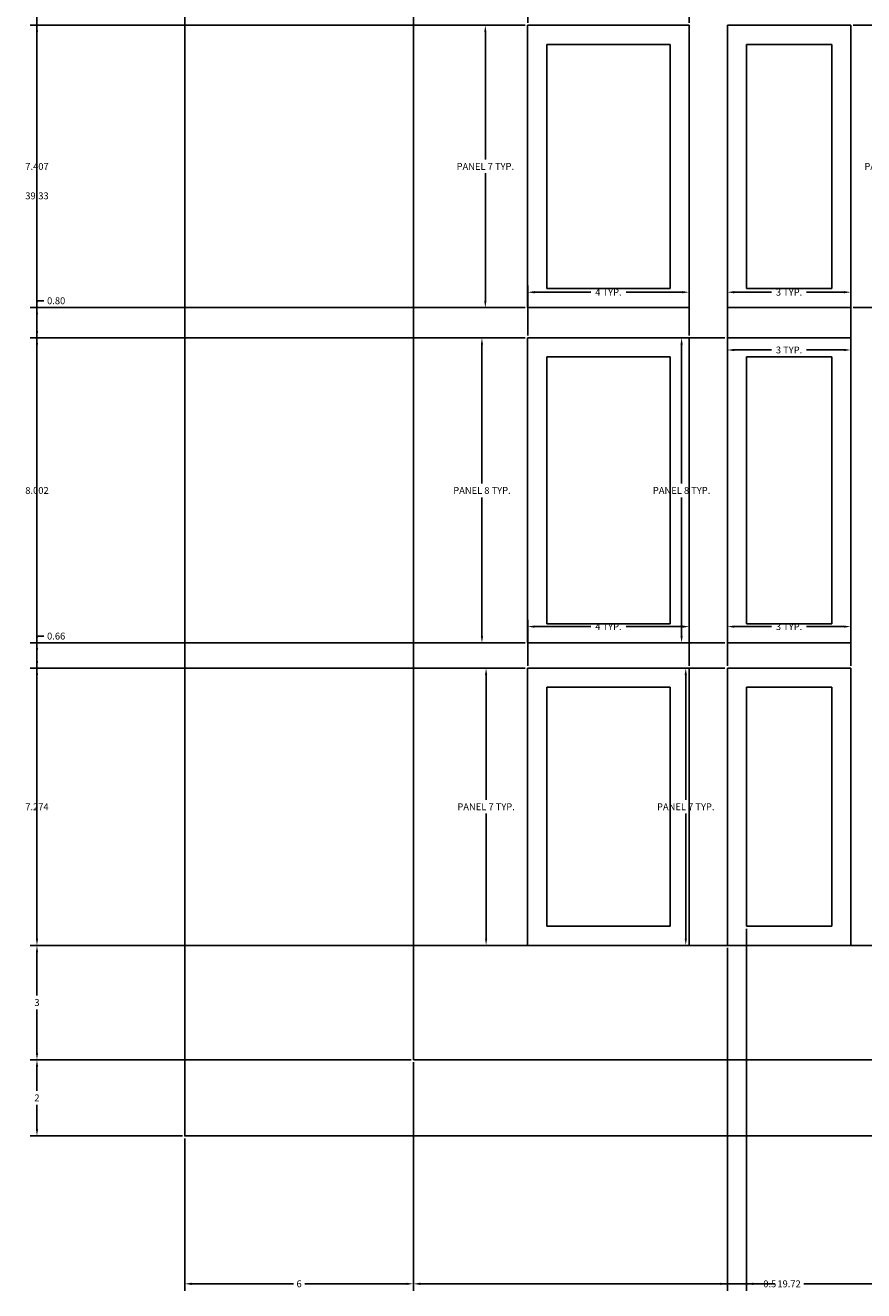
# Model space of a CAD drawing. Units: inches. Extents: x 12532.3 to 12594.9, y 6967.5 to 7063.
# Tile 1 of 9: x 12532.3 to 12554.3, y 6967.5 to 7000.7. Entities that reach past the tile are written whole.
import ezdxf

# ---------------------------------------------------------------- set-up
doc = ezdxf.new("R2010")
doc.units = ezdxf.units.IN
doc.header["$MEASUREMENT"] = 0
doc.header["$PDMODE"] = 98
doc.layers.add('A-ANNO-DIMS', color=2, linetype='Continuous', lineweight=18)
doc.layers.add('A-DOOR', color=4, linetype='Continuous', lineweight=25)
doc.styles.get("Standard").update_dxf_attribs({"font": 'arial.ttf'})
doc.dimstyles.get("Standard").update_dxf_attribs({"dimtxt": 0.18, "dimasz": 0.18, "dimexe": 0.18, "dimexo": 0.0625, "dimgap": 0.09, "dimtad": 0, "dimtih": 1, "dimtoh": 1, "dimdec": 4, "dimzin": 0, "dimdsep": 46, "dimtxsty": 'Standard', "dimcen": 0.09, "dimadec": 0, "dimazin": 0, "dimtfac": 1, "dimtdec": 4, "dimtofl": 0, "dimtmove": 0, "dimatfit": 3, "dimfxl": 1, "dimtolj": 1, "dimtzin": 0, "dimarcsym": 0})

# ---------------------------------------------------------------- blocks, each defined once
blk = doc.blocks.new('DOOR-PANEL-3_2x7_3')
for p, q in [((0, 7.273), (0, 0)), ((0, 7.273), (3.24, 7.273)), ((3.24, 7.273), (3.24, 0)), ((0.5, 6.773), (0.5, 0.5)), ((0.5, 6.773), (2.74, 6.773)), ((2.74, 6.773), (2.74, 0.5)), ((2.74, 0.5), (0.5, 0.5)), ((3.24, 0), (0, 0))]:
    blk.add_line(p, q)
blk = doc.blocks.new('DOOR-PANEL-4_2x7_3')
for p, q in [((0, 7.273), (0, 0)), ((0, 7.273), (4.241, 7.273)), ((4.241, 7.273), (4.241, 0)), ((0.5, 6.773), (0.5, 0.5)), ((0.5, 6.773), (3.741, 6.773)), ((3.741, 6.773), (3.741, 0.5)), ((3.741, 0.5), (0.5, 0.5)), ((4.241, 0), (0, 0))]:
    blk.add_line(p, q)
blk = doc.blocks.new('DOOR-PANEL-4_2x7_4')
for p, q in [((4.241, 7.408), (0, 7.408)), ((0, 7.408), (0, 0)), ((4.241, 7.408), (4.241, 0)), ((3.741, 6.908), (0.5, 6.908)), ((0.5, 6.908), (0.5, 0.5)), ((3.741, 6.908), (3.741, 0.5)), ((3.741, 0.5), (0.5, 0.5)), ((4.241, 0), (0, 0))]:
    blk.add_line(p, q)
blk = doc.blocks.new('DOOR-PANEL-4_2x8_0')
for p, q in [((4.241, 8.003), (0, 8.003)), ((0, 8.003), (0, 0)), ((4.241, 8.003), (4.241, 0)), ((3.741, 7.503), (0.5, 7.503)), ((0.5, 7.503), (0.5, 0.5)), ((3.741, 7.503), (3.741, 0.5)), ((3.741, 0.5), (0.5, 0.5)), ((4.241, 0), (0, 0))]:
    blk.add_line(p, q)
blk = doc.blocks.new('DOOR-PANEL-3_2x8_0')
for p, q in [((3.24, 8.003), (0, 8.003)), ((0, 8.003), (0, 0)), ((3.24, 8.003), (3.24, 0)), ((2.74, 7.503), (0.5, 7.503)), ((0.5, 7.503), (0.5, 0.5)), ((2.74, 7.503), (2.74, 0.5)), ((2.74, 0.5), (0.5, 0.5)), ((3.24, 0), (0, 0))]:
    blk.add_line(p, q)
blk = doc.blocks.new('DOOR-PANEL-3_2x7_4')
for p, q in [((0, 0), (0, 7.408)), ((0, 7.408), (3.24, 7.408)), ((3.24, 0), (3.24, 7.408)), ((0.5, 0.5), (0.5, 6.908)), ((0.5, 6.908), (2.74, 6.908)), ((2.74, 0.5), (2.74, 6.908)), ((0.5, 0.5), (2.74, 0.5)), ((0, 0), (3.24, 0))]:
    blk.add_line(p, q)
blk = doc.blocks.new('*D11')
at = {"layer": 'A-ANNO-DIMS', "color": 0, "lineweight": -2, "transparency": 16777216}
for p, q in [((12545.388, 6983.87), (12544.179, 6983.87)), ((12544.359, 6983.69), (12544.359, 6980.414)), ((12544.359, 6976.777), (12544.359, 6980.053)), ((12545.388, 6976.597), (12544.179, 6976.597))]:
    blk.add_line(p, q, dxfattribs=at)
at = {"layer": 'A-ANNO-DIMS', "color": 0, "transparency": 16777216}
for points in [[(12544.329, 6983.69), (12544.389, 6983.69), (12544.359, 6983.87)], [(12544.329, 6976.777), (12544.389, 6976.777), (12544.359, 6976.597)]]:
    blk.add_solid(points, dxfattribs=at)
at = {"layer": 'Defpoints', "color": 0, "transparency": 16777216}
for p in [(12545.45, 6983.87), (12544.359, 6976.597), (12545.45, 6976.597)]:
    blk.add_point(p, dxfattribs=at)
at = {"layer": 'A-ANNO-DIMS', "color": 0, "transparency": 16777216, "insert": (12544.359, 6980.234), "char_height": 0.18, "attachment_point": 5}
blk.add_mtext('\\A1;PANEL 7 TYP.', dxfattribs=at)
blk = doc.blocks.new('*D12')
at = {"layer": 'A-ANNO-DIMS', "color": 0, "lineweight": -2, "transparency": 16777216}
for p, q in [((12545.45, 6983.933), (12545.45, 6985.141)), ((12549.691, 6983.933), (12549.691, 6985.141)), ((12545.63, 6984.961), (12547.109, 6984.961)), ((12549.511, 6984.961), (12548.032, 6984.961))]:
    blk.add_line(p, q, dxfattribs=at)
at = {"layer": 'A-ANNO-DIMS', "color": 0, "transparency": 16777216}
for points in [[(12545.63, 6984.991), (12545.63, 6984.931), (12545.45, 6984.961)], [(12549.511, 6984.991), (12549.511, 6984.931), (12549.691, 6984.961)]]:
    blk.add_solid(points, dxfattribs=at)
at = {"layer": 'Defpoints', "color": 0, "transparency": 16777216}
for p in [(12545.45, 6984.961), (12545.45, 6983.87), (12549.691, 6983.87)]:
    blk.add_point(p, dxfattribs=at)
at = {"layer": 'A-ANNO-DIMS', "color": 0, "transparency": 16777216, "insert": (12547.57, 6984.961), "char_height": 0.18, "attachment_point": 5}
blk.add_mtext('\\A1;4 TYP.', dxfattribs=at)
blk = doc.blocks.new('*D17')
at = {"layer": 'A-ANNO-DIMS', "color": 0, "lineweight": -2, "transparency": 16777216}
for p, q in [((12545.388, 7000.738), (12544.159, 7000.738)), ((12544.339, 7000.558), (12544.339, 6997.214)), ((12544.339, 6993.51), (12544.339, 6996.854)), ((12545.388, 6993.33), (12544.159, 6993.33))]:
    blk.add_line(p, q, dxfattribs=at)
at = {"layer": 'A-ANNO-DIMS', "color": 0, "transparency": 16777216}
for points in [[(12544.309, 7000.558), (12544.369, 7000.558), (12544.339, 7000.738)], [(12544.309, 6993.51), (12544.369, 6993.51), (12544.339, 6993.33)]]:
    blk.add_solid(points, dxfattribs=at)
at = {"layer": 'Defpoints', "color": 0, "transparency": 16777216}
for p in [(12545.45, 7000.738), (12544.339, 6993.33), (12545.45, 6993.33)]:
    blk.add_point(p, dxfattribs=at)
at = {"layer": 'A-ANNO-DIMS', "color": 0, "transparency": 16777216, "insert": (12544.339, 6997.034), "char_height": 0.18, "attachment_point": 5}
blk.add_mtext('\\A1;PANEL 7 TYP.', dxfattribs=at)
blk = doc.blocks.new('*D18')
at = {"layer": 'A-ANNO-DIMS', "color": 0, "lineweight": -2, "transparency": 16777216}
for p, q in [((12545.45, 7000.8), (12545.45, 7002.029)), ((12545.63, 7001.849), (12547.109, 7001.849)), ((12549.511, 7001.849), (12548.032, 7001.849)), ((12549.691, 7000.8), (12549.691, 7002.029))]:
    blk.add_line(p, q, dxfattribs=at)
at = {"layer": 'A-ANNO-DIMS', "color": 0, "transparency": 16777216}
for points in [[(12545.63, 7001.879), (12545.63, 7001.819), (12545.45, 7001.849)], [(12549.511, 7001.879), (12549.511, 7001.819), (12549.691, 7001.849)]]:
    blk.add_solid(points, dxfattribs=at)
at = {"layer": 'Defpoints', "color": 0, "transparency": 16777216}
for p in [(12545.45, 7001.849), (12545.45, 7000.738), (12549.691, 7000.738)]:
    blk.add_point(p, dxfattribs=at)
at = {"layer": 'A-ANNO-DIMS', "color": 0, "transparency": 16777216, "insert": (12547.57, 7001.849), "char_height": 0.18, "attachment_point": 5}
blk.add_mtext('\\A1;4 TYP.', dxfattribs=at)
blk = doc.blocks.new('*D19')
at = {"layer": 'A-ANNO-DIMS', "color": 0, "lineweight": -2, "transparency": 16777216}
for p, q in [((12545.388, 6992.535), (12544.07, 6992.535)), ((12544.25, 6992.355), (12544.25, 6988.715)), ((12544.25, 6984.712), (12544.25, 6988.352)), ((12545.388, 6984.532), (12544.07, 6984.532))]:
    blk.add_line(p, q, dxfattribs=at)
at = {"layer": 'A-ANNO-DIMS', "color": 0, "transparency": 16777216}
for points in [[(12544.22, 6992.355), (12544.28, 6992.355), (12544.25, 6992.535)], [(12544.22, 6984.712), (12544.28, 6984.712), (12544.25, 6984.532)]]:
    blk.add_solid(points, dxfattribs=at)
at = {"layer": 'Defpoints', "color": 0, "transparency": 16777216}
for p in [(12545.45, 6992.535), (12544.25, 6984.532), (12545.45, 6984.532)]:
    blk.add_point(p, dxfattribs=at)
at = {"layer": 'A-ANNO-DIMS', "color": 0, "transparency": 16777216, "insert": (12544.25, 6988.534), "char_height": 0.18, "attachment_point": 5}
blk.add_mtext('\\A1;PANEL 8 TYP.', dxfattribs=at)
blk = doc.blocks.new('*D20')
at = {"layer": 'A-ANNO-DIMS', "color": 0, "lineweight": -2, "transparency": 16777216}
for p, q in [((12545.45, 6992.597), (12545.45, 6993.915)), ((12549.691, 6992.597), (12549.691, 6993.915)), ((12545.63, 6993.735), (12547.109, 6993.735)), ((12549.511, 6993.735), (12548.032, 6993.735))]:
    blk.add_line(p, q, dxfattribs=at)
at = {"layer": 'A-ANNO-DIMS', "color": 0, "transparency": 16777216}
for points in [[(12545.63, 6993.765), (12545.63, 6993.705), (12545.45, 6993.735)], [(12549.511, 6993.765), (12549.511, 6993.705), (12549.691, 6993.735)]]:
    blk.add_solid(points, dxfattribs=at)
at = {"layer": 'Defpoints', "color": 0, "transparency": 16777216}
for p in [(12545.45, 6993.735), (12545.45, 6992.535), (12549.691, 6992.535)]:
    blk.add_point(p, dxfattribs=at)
at = {"layer": 'A-ANNO-DIMS', "color": 0, "transparency": 16777216, "insert": (12547.57, 6993.735), "char_height": 0.18, "attachment_point": 5}
blk.add_mtext('\\A1;4 TYP.', dxfattribs=at)
blk = doc.blocks.new('*D21')
at = {"layer": 'A-ANNO-DIMS', "color": 0, "lineweight": -2, "transparency": 16777216}
for p, q in [((12550.628, 6983.87), (12549.42, 6983.87)), ((12549.6, 6983.69), (12549.6, 6980.414)), ((12549.6, 6976.777), (12549.6, 6980.053)), ((12550.628, 6976.597), (12549.42, 6976.597))]:
    blk.add_line(p, q, dxfattribs=at)
at = {"layer": 'A-ANNO-DIMS', "color": 0, "transparency": 16777216}
for points in [[(12549.57, 6983.69), (12549.63, 6983.69), (12549.6, 6983.87)], [(12549.57, 6976.777), (12549.63, 6976.777), (12549.6, 6976.597)]]:
    blk.add_solid(points, dxfattribs=at)
at = {"layer": 'Defpoints', "color": 0, "transparency": 16777216}
for p in [(12550.691, 6983.87), (12549.6, 6976.597), (12550.691, 6976.597)]:
    blk.add_point(p, dxfattribs=at)
at = {"layer": 'A-ANNO-DIMS', "color": 0, "transparency": 16777216, "insert": (12549.6, 6980.234), "char_height": 0.18, "attachment_point": 5}
blk.add_mtext('\\A1;PANEL 7 TYP.', dxfattribs=at)
blk = doc.blocks.new('*D22')
at = {"layer": 'A-ANNO-DIMS', "color": 0, "lineweight": -2, "transparency": 16777216}
for p, q in [((12550.691, 6983.933), (12550.691, 6985.141)), ((12553.931, 6983.933), (12553.931, 6985.141)), ((12550.871, 6984.961), (12551.853, 6984.961)), ((12553.751, 6984.961), (12552.769, 6984.961))]:
    blk.add_line(p, q, dxfattribs=at)
at = {"layer": 'A-ANNO-DIMS', "color": 0, "transparency": 16777216}
for points in [[(12550.871, 6984.991), (12550.871, 6984.931), (12550.691, 6984.961)], [(12553.751, 6984.991), (12553.751, 6984.931), (12553.931, 6984.961)]]:
    blk.add_solid(points, dxfattribs=at)
at = {"layer": 'Defpoints', "color": 0, "transparency": 16777216}
for p in [(12550.691, 6984.961), (12550.691, 6983.87), (12553.931, 6983.87)]:
    blk.add_point(p, dxfattribs=at)
at = {"layer": 'A-ANNO-DIMS', "color": 0, "transparency": 16777216, "insert": (12552.311, 6984.961), "char_height": 0.18, "attachment_point": 5}
blk.add_mtext('\\A1;3 TYP.', dxfattribs=at)
blk = doc.blocks.new('*D23')
at = {"layer": 'A-ANNO-DIMS', "color": 0, "lineweight": -2, "transparency": 16777216}
for p, q in [((12550.628, 6992.535), (12549.31, 6992.535)), ((12549.49, 6992.355), (12549.49, 6988.715)), ((12549.49, 6984.712), (12549.49, 6988.352)), ((12550.628, 6984.532), (12549.31, 6984.532))]:
    blk.add_line(p, q, dxfattribs=at)
at = {"layer": 'A-ANNO-DIMS', "color": 0, "transparency": 16777216}
for points in [[(12549.46, 6992.355), (12549.52, 6992.355), (12549.49, 6992.535)], [(12549.46, 6984.712), (12549.52, 6984.712), (12549.49, 6984.532)]]:
    blk.add_solid(points, dxfattribs=at)
at = {"layer": 'Defpoints', "color": 0, "transparency": 16777216}
for p in [(12550.691, 6992.535), (12549.49, 6984.532), (12550.691, 6984.532)]:
    blk.add_point(p, dxfattribs=at)
at = {"layer": 'A-ANNO-DIMS', "color": 0, "transparency": 16777216, "insert": (12549.49, 6988.534), "char_height": 0.18, "attachment_point": 5}
blk.add_mtext('\\A1;PANEL 8 TYP.', dxfattribs=at)
blk = doc.blocks.new('*D24')
at = {"layer": 'A-ANNO-DIMS', "color": 0, "lineweight": -2, "transparency": 16777216}
for p, q in [((12550.691, 6992.597), (12550.691, 6993.915)), ((12553.931, 6992.597), (12553.931, 6993.915)), ((12550.871, 6993.735), (12551.853, 6993.735)), ((12553.751, 6993.735), (12552.769, 6993.735))]:
    blk.add_line(p, q, dxfattribs=at)
at = {"layer": 'A-ANNO-DIMS', "color": 0, "transparency": 16777216}
for points in [[(12550.871, 6993.765), (12550.871, 6993.705), (12550.691, 6993.735)], [(12553.751, 6993.765), (12553.751, 6993.705), (12553.931, 6993.735)]]:
    blk.add_solid(points, dxfattribs=at)
at = {"layer": 'Defpoints', "color": 0, "transparency": 16777216}
for p in [(12550.691, 6993.735), (12550.691, 6992.535), (12553.931, 6992.535)]:
    blk.add_point(p, dxfattribs=at)
at = {"layer": 'A-ANNO-DIMS', "color": 0, "transparency": 16777216, "insert": (12552.311, 6993.735), "char_height": 0.18, "attachment_point": 5}
blk.add_mtext('\\A1;3 TYP.', dxfattribs=at)
blk = doc.blocks.new('*D25')
at = {"layer": 'A-ANNO-DIMS', "color": 0, "lineweight": -2, "transparency": 16777216}
for p, q in [((12553.994, 7000.738), (12555.223, 7000.738)), ((12555.043, 7000.558), (12555.043, 6997.214)), ((12555.043, 6993.51), (12555.043, 6996.854)), ((12553.994, 6993.33), (12555.223, 6993.33))]:
    blk.add_line(p, q, dxfattribs=at)
at = {"layer": 'A-ANNO-DIMS', "color": 0, "transparency": 16777216}
for points in [[(12555.013, 7000.558), (12555.073, 7000.558), (12555.043, 7000.738)], [(12555.013, 6993.51), (12555.073, 6993.51), (12555.043, 6993.33)]]:
    blk.add_solid(points, dxfattribs=at)
at = {"layer": 'Defpoints', "color": 0, "transparency": 16777216}
for p in [(12553.931, 7000.738), (12555.043, 7000.738), (12553.931, 6993.33)]:
    blk.add_point(p, dxfattribs=at)
at = {"layer": 'A-ANNO-DIMS', "color": 0, "transparency": 16777216, "insert": (12555.043, 6997.034), "char_height": 0.18, "attachment_point": 5}
blk.add_mtext('\\A1;PANEL 7 TYP.', dxfattribs=at)
blk = doc.blocks.new('*D26')
at = {"layer": 'A-ANNO-DIMS', "color": 0, "lineweight": -2, "transparency": 16777216}
for p, q in [((12550.691, 6993.268), (12550.691, 6992.039)), ((12553.931, 6993.268), (12553.931, 6992.039)), ((12550.871, 6992.219), (12551.853, 6992.219)), ((12553.751, 6992.219), (12552.769, 6992.219))]:
    blk.add_line(p, q, dxfattribs=at)
at = {"layer": 'A-ANNO-DIMS', "color": 0, "transparency": 16777216}
for points in [[(12550.871, 6992.249), (12550.871, 6992.189), (12550.691, 6992.219)], [(12553.751, 6992.249), (12553.751, 6992.189), (12553.931, 6992.219)]]:
    blk.add_solid(points, dxfattribs=at)
at = {"layer": 'Defpoints', "color": 0, "transparency": 16777216}
for p in [(12550.691, 6993.33), (12553.931, 6993.33), (12553.931, 6992.219)]:
    blk.add_point(p, dxfattribs=at)
at = {"layer": 'A-ANNO-DIMS', "color": 0, "transparency": 16777216, "insert": (12552.311, 6992.219), "char_height": 0.18, "attachment_point": 5}
blk.add_mtext('\\A1;3 TYP.', dxfattribs=at)
blk = doc.blocks.new('*D34')
at = {"layer": 'A-ANNO-DIMS', "color": 0, "lineweight": -2, "transparency": 16777216}
for p, q in [((12542.450147, 6973.534253), (12542.450147, 6967.536753)), ((12536.450147, 6971.534253), (12536.450147, 6967.536753)), ((12536.630147, 6967.716753), (12539.30072, 6967.716753)), ((12542.270147, 6967.716753), (12539.599574, 6967.716753))]:
    blk.add_line(p, q, dxfattribs=at)
at = {"layer": 'A-ANNO-DIMS', "color": 0, "transparency": 16777216}
for points in [[(12536.630147, 6967.746753), (12536.630147, 6967.686753), (12536.450147, 6967.716753)], [(12542.270147, 6967.746753), (12542.270147, 6967.686753), (12542.450147, 6967.716753)]]:
    blk.add_solid(points, dxfattribs=at)
at = {"layer": 'Defpoints', "color": 0, "transparency": 16777216}
for p in [(12542.450147, 6973.596753), (12536.450147, 6971.596753), (12542.450147, 6967.716753)]:
    blk.add_point(p, dxfattribs=at)
at = {"layer": 'A-ANNO-DIMS', "color": 0, "transparency": 16777216, "insert": (12539.450147, 6967.716753), "char_height": 0.18, "attachment_point": 5}
blk.add_mtext('\\A1;6', dxfattribs=at)
blk = doc.blocks.new('*D35')
at = {"layer": 'A-ANNO-DIMS', "color": 0, "lineweight": -2, "transparency": 16777216}
for p, q in [((12542.45, 6973.534), (12542.45, 6967.537)), ((12562.172, 6973.534), (12562.172, 6967.537)), ((12542.63, 6967.717), (12551.927, 6967.717)), ((12561.992, 6967.717), (12552.695, 6967.717))]:
    blk.add_line(p, q, dxfattribs=at)
at = {"layer": 'A-ANNO-DIMS', "color": 0, "transparency": 16777216}
for points in [[(12542.63, 6967.747), (12542.63, 6967.687), (12542.45, 6967.717)], [(12561.992, 6967.747), (12561.992, 6967.687), (12562.172, 6967.717)]]:
    blk.add_solid(points, dxfattribs=at)
at = {"layer": 'Defpoints', "color": 0, "transparency": 16777216}
for p in [(12542.45, 6973.597), (12562.172, 6973.597), (12562.172, 6967.717)]:
    blk.add_point(p, dxfattribs=at)
at = {"layer": 'A-ANNO-DIMS', "color": 0, "transparency": 16777216, "insert": (12552.311, 6967.717), "char_height": 0.18, "attachment_point": 5}
blk.add_mtext('\\A1;19.72', dxfattribs=at)
blk = doc.blocks.new('*D41')
at = {"layer": 'A-ANNO-DIMS', "color": 0, "lineweight": -2, "transparency": 16777216}
for p, q in [((12542.388, 6973.597), (12532.39, 6973.597)), ((12532.57, 6973.417), (12532.57, 6972.777)), ((12532.57, 6971.777), (12532.57, 6972.416)), ((12536.388, 6971.597), (12532.39, 6971.597))]:
    blk.add_line(p, q, dxfattribs=at)
at = {"layer": 'A-ANNO-DIMS', "color": 0, "transparency": 16777216}
for points in [[(12532.54, 6973.417), (12532.6, 6973.417), (12532.57, 6973.597)], [(12532.54, 6971.777), (12532.6, 6971.777), (12532.57, 6971.597)]]:
    blk.add_solid(points, dxfattribs=at)
at = {"layer": 'Defpoints', "color": 0, "transparency": 16777216}
for p in [(12532.57, 6973.597), (12542.45, 6973.597), (12536.45, 6971.597)]:
    blk.add_point(p, dxfattribs=at)
at = {"layer": 'A-ANNO-DIMS', "color": 0, "transparency": 16777216, "insert": (12532.57, 6972.597), "char_height": 0.18, "attachment_point": 5}
blk.add_mtext('\\A1;2', dxfattribs=at)
blk = doc.blocks.new('*D42')
at = {"layer": 'A-ANNO-DIMS', "color": 0, "lineweight": -2, "transparency": 16777216}
for p, q in [((12545.388, 6976.597), (12532.39, 6976.597)), ((12532.57, 6976.417), (12532.57, 6975.279)), ((12532.57, 6973.777), (12532.57, 6974.915)), ((12542.388, 6973.597), (12532.39, 6973.597))]:
    blk.add_line(p, q, dxfattribs=at)
at = {"layer": 'A-ANNO-DIMS', "color": 0, "transparency": 16777216}
for points in [[(12532.54, 6976.417), (12532.6, 6976.417), (12532.57, 6976.597)], [(12532.54, 6973.777), (12532.6, 6973.777), (12532.57, 6973.597)]]:
    blk.add_solid(points, dxfattribs=at)
at = {"layer": 'Defpoints', "color": 0, "transparency": 16777216}
for p in [(12532.57, 6976.597), (12545.45, 6976.597), (12542.45, 6973.597)]:
    blk.add_point(p, dxfattribs=at)
at = {"layer": 'A-ANNO-DIMS', "color": 0, "transparency": 16777216, "insert": (12532.57, 6975.097), "char_height": 0.18, "attachment_point": 5}
blk.add_mtext('\\A1;3', dxfattribs=at)
blk = doc.blocks.new('*D43')
at = {"layer": 'A-ANNO-DIMS', "color": 0, "lineweight": -2, "transparency": 16777216}
for p, q in [((12566.11, 7015.929), (12532.39, 7015.929)), ((12532.57, 7015.749), (12532.57, 6996.445)), ((12532.57, 6976.777), (12532.57, 6996.081)), ((12566.11, 6976.597), (12532.39, 6976.597))]:
    blk.add_line(p, q, dxfattribs=at)
at = {"layer": 'A-ANNO-DIMS', "color": 0, "transparency": 16777216}
for points in [[(12532.54, 7015.749), (12532.6, 7015.749), (12532.57, 7015.929)], [(12532.54, 6976.777), (12532.6, 6976.777), (12532.57, 6976.597)]]:
    blk.add_solid(points, dxfattribs=at)
at = {"layer": 'Defpoints', "color": 0, "transparency": 16777216}
for p in [(12532.57, 7015.929), (12566.172, 7015.929), (12566.172, 6976.597)]:
    blk.add_point(p, dxfattribs=at)
at = {"layer": 'A-ANNO-DIMS', "color": 0, "transparency": 16777216, "insert": (12532.57, 6996.263), "char_height": 0.18, "attachment_point": 5}
blk.add_mtext('\\A1;39.33', dxfattribs=at)
blk = doc.blocks.new('*D51')
at = {"layer": 'A-ANNO-DIMS', "color": 0, "lineweight": -2, "transparency": 16777216}
for p, q in [((12545.388, 6983.87), (12532.39, 6983.87)), ((12532.57, 6983.69), (12532.57, 6980.414)), ((12532.57, 6976.777), (12532.57, 6980.053)), ((12545.388, 6976.597), (12532.39, 6976.597))]:
    blk.add_line(p, q, dxfattribs=at)
at = {"layer": 'A-ANNO-DIMS', "color": 0, "transparency": 16777216}
for points in [[(12532.54, 6983.69), (12532.6, 6983.69), (12532.57, 6983.87)], [(12532.54, 6976.777), (12532.6, 6976.777), (12532.57, 6976.597)]]:
    blk.add_solid(points, dxfattribs=at)
at = {"layer": 'Defpoints', "color": 0, "transparency": 16777216}
for p in [(12532.57, 6983.87), (12545.45, 6983.87), (12545.45, 6976.597)]:
    blk.add_point(p, dxfattribs=at)
at = {"layer": 'A-ANNO-DIMS', "color": 0, "transparency": 16777216, "insert": (12532.57, 6980.234), "char_height": 0.18, "attachment_point": 5}
blk.add_mtext('\\A1;7.274', dxfattribs=at)
blk = doc.blocks.new('*D52')
at = {"layer": 'A-ANNO-DIMS', "color": 0, "lineweight": -2, "transparency": 16777216}
for p, q in [((12545.388, 6984.532), (12532.39, 6984.532)), ((12532.57, 6984.532), (12532.57, 6984.712)), ((12532.57, 6984.712), (12532.75, 6984.712)), ((12532.57, 6984.05), (12532.57, 6984.352)), ((12545.388, 6983.87), (12532.39, 6983.87))]:
    blk.add_line(p, q, dxfattribs=at)
at = {"layer": 'A-ANNO-DIMS', "color": 0, "transparency": 16777216}
for points in [[(12532.54, 6984.352), (12532.6, 6984.352), (12532.57, 6984.532)], [(12532.54, 6984.05), (12532.6, 6984.05), (12532.57, 6983.87)]]:
    blk.add_solid(points, dxfattribs=at)
at = {"layer": 'Defpoints', "color": 0, "transparency": 16777216}
for p in [(12532.57, 6984.532), (12545.45, 6984.532), (12545.45, 6983.87)]:
    blk.add_point(p, dxfattribs=at)
at = {"layer": 'A-ANNO-DIMS', "color": 0, "transparency": 16777216, "insert": (12533.074, 6984.712), "char_height": 0.18, "attachment_point": 5}
blk.add_mtext('\\A1;0.66', dxfattribs=at)
blk = doc.blocks.new('*D53')
at = {"layer": 'A-ANNO-DIMS', "color": 0, "lineweight": -2, "transparency": 16777216}
for p, q in [((12545.388, 6992.535), (12532.39, 6992.535)), ((12532.57, 6992.355), (12532.57, 6988.715)), ((12532.57, 6984.712), (12532.57, 6988.352)), ((12545.388, 6984.532), (12532.39, 6984.532))]:
    blk.add_line(p, q, dxfattribs=at)
at = {"layer": 'A-ANNO-DIMS', "color": 0, "transparency": 16777216}
for points in [[(12532.54, 6992.355), (12532.6, 6992.355), (12532.57, 6992.535)], [(12532.54, 6984.712), (12532.6, 6984.712), (12532.57, 6984.532)]]:
    blk.add_solid(points, dxfattribs=at)
at = {"layer": 'Defpoints', "color": 0, "transparency": 16777216}
for p in [(12532.57, 6992.535), (12545.45, 6992.535), (12545.45, 6984.532)]:
    blk.add_point(p, dxfattribs=at)
at = {"layer": 'A-ANNO-DIMS', "color": 0, "transparency": 16777216, "insert": (12532.57, 6988.534), "char_height": 0.18, "attachment_point": 5}
blk.add_mtext('\\A1;8.002', dxfattribs=at)
blk = doc.blocks.new('*D54')
at = {"layer": 'A-ANNO-DIMS', "color": 0, "lineweight": -2, "transparency": 16777216}
for p, q in [((12532.57, 6993.33), (12532.57, 6993.51)), ((12532.57, 6993.51), (12532.75, 6993.51)), ((12545.388, 6993.33), (12532.39, 6993.33)), ((12532.57, 6992.715), (12532.57, 6993.15)), ((12545.388, 6992.535), (12532.39, 6992.535))]:
    blk.add_line(p, q, dxfattribs=at)
at = {"layer": 'A-ANNO-DIMS', "color": 0, "transparency": 16777216}
for points in [[(12532.54, 6993.15), (12532.6, 6993.15), (12532.57, 6993.33)], [(12532.54, 6992.715), (12532.6, 6992.715), (12532.57, 6992.535)]]:
    blk.add_solid(points, dxfattribs=at)
at = {"layer": 'Defpoints', "color": 0, "transparency": 16777216}
for p in [(12532.57, 6993.33), (12545.45, 6993.33), (12545.45, 6992.535)]:
    blk.add_point(p, dxfattribs=at)
at = {"layer": 'A-ANNO-DIMS', "color": 0, "transparency": 16777216, "insert": (12533.074, 6993.51), "char_height": 0.18, "attachment_point": 5}
blk.add_mtext('\\A1;0.80', dxfattribs=at)
blk = doc.blocks.new('*D55')
at = {"layer": 'A-ANNO-DIMS', "color": 0, "lineweight": -2, "transparency": 16777216}
for p, q in [((12545.388, 7000.738), (12532.39, 7000.738)), ((12532.57, 7000.558), (12532.57, 6997.216)), ((12532.57, 6993.51), (12532.57, 6996.852)), ((12545.388, 6993.33), (12532.39, 6993.33))]:
    blk.add_line(p, q, dxfattribs=at)
at = {"layer": 'A-ANNO-DIMS', "color": 0, "transparency": 16777216}
for points in [[(12532.54, 7000.558), (12532.6, 7000.558), (12532.57, 7000.738)], [(12532.54, 6993.51), (12532.6, 6993.51), (12532.57, 6993.33)]]:
    blk.add_solid(points, dxfattribs=at)
at = {"layer": 'Defpoints', "color": 0, "transparency": 16777216}
for p in [(12532.57, 7000.738), (12545.45, 7000.738), (12545.45, 6993.33)]:
    blk.add_point(p, dxfattribs=at)
at = {"layer": 'A-ANNO-DIMS', "color": 0, "transparency": 16777216, "insert": (12532.57, 6997.034), "char_height": 0.18, "attachment_point": 5}
blk.add_mtext('\\A1;7.407', dxfattribs=at)
blk = doc.blocks.new('*D60')
at = {"layer": 'A-ANNO-DIMS', "color": 0, "lineweight": -2, "transparency": 16777216}
for p, q in [((12551.191, 6977.034), (12551.191, 6967.537)), ((12550.691, 6976.534), (12550.691, 6967.537)), ((12550.511, 6967.717), (12550.331, 6967.717)), ((12551.371, 6967.717), (12551.551, 6967.717))]:
    blk.add_line(p, q, dxfattribs=at)
at = {"layer": 'A-ANNO-DIMS', "color": 0, "transparency": 16777216}
for points in [[(12550.511, 6967.747), (12550.511, 6967.687), (12550.691, 6967.717)], [(12551.371, 6967.747), (12551.371, 6967.687), (12551.191, 6967.717)]]:
    blk.add_solid(points, dxfattribs=at)
at = {"layer": 'Defpoints', "color": 0, "transparency": 16777216}
for p in [(12551.191, 6977.097), (12550.691, 6976.597), (12551.191, 6967.717)]:
    blk.add_point(p, dxfattribs=at)
at = {"layer": 'A-ANNO-DIMS', "color": 0, "transparency": 16777216, "insert": (12551.805, 6967.717), "char_height": 0.18, "attachment_point": 5}
blk.add_mtext('\\A1;0.5', dxfattribs=at)

msp = doc.modelspace()

# ---------------------------------------------------------------- linework, layer by layer
at = {"layer": 'A-DOOR'}
msp.add_lwpolyline([(12536.4501, 7020.9287), (12588.894, 7020.9287), (12588.894, 6971.5968), (12536.4501, 6971.5968)], close=True, dxfattribs=at)
for points in [[(12542.4501, 6973.5968), (12542.4501, 7018.9287)], [(12582.894, 6973.5968), (12542.4501, 6973.5968)]]:
    msp.add_lwpolyline(points, dxfattribs=at)

# ---------------------------------------------------------------- block references
at = {"layer": 'A-DOOR', "rotation": 180}
for name, p in [('DOOR-PANEL-4_2x7_4', (12549.6909, 7000.738)), ('DOOR-PANEL-4_2x8_0', (12549.6909, 6992.535)), ('DOOR-PANEL-3_2x8_0', (12553.9312, 6992.535)), ('DOOR-PANEL-4_2x7_3', (12549.6909, 6983.87)), ('DOOR-PANEL-3_2x7_3', (12553.9312, 6983.87))]:
    msp.add_blockref(name, p, dxfattribs=at)
at = {"layer": 'A-DOOR'}
msp.add_blockref('DOOR-PANEL-3_2x7_4', (12550.691, 6993.33), dxfattribs=at)

# ---------------------------------------------------------------- dimensions: what is measured, and where the dimension line sits
at = {"layer": 'A-ANNO-DIMS'}
for base, p1, p2, override, picture, middle in [((12532.5701, 7015.9287), (12566.1721, 6976.5968), (12566.1721, 7015.9287), {"dimdec": 2, "dimlfac": 1, "dimrnd": 0, "dimzin": 0, "dimdsep": 46, "dimlunit": 2}, '*D43', (12532.5701, 6996.2627)), ((12532.5701, 7000.7376), (12545.4501, 6993.3303), (12545.4501, 7000.7376), {"dimdec": 3, "dimlfac": 1, "dimrnd": 0, "dimzin": 0, "dimdsep": 46, "dimlunit": 2}, '*D55', (12532.5701, 6997.034)), ((12532.5701, 6993.3303), (12545.4501, 6992.5346), (12545.4501, 6993.3303), {"dimdec": 2, "dimlfac": 1, "dimrnd": 0, "dimzin": 0, "dimdsep": 46, "dimlunit": 2}, '*D54', (12533.0736, 6993.5103)), ((12532.5701, 6992.5346), (12545.4501, 6984.5324), (12545.4501, 6992.5346), {"dimdec": 3, "dimlfac": 1, "dimrnd": 0, "dimzin": 0, "dimdsep": 46, "dimlunit": 2}, '*D53', (12532.5701, 6988.5335)), ((12532.5701, 6984.5324), (12545.4501, 6983.8703), (12545.4501, 6984.5324), {"dimdec": 2, "dimlfac": 1, "dimrnd": 0, "dimzin": 0, "dimdsep": 46, "dimlunit": 2}, '*D52', (12533.0739, 6984.7124)), ((12532.570147, 6983.870254), (12545.450147, 6976.596753), (12545.450147, 6983.870254), {"dimdec": 3, "dimlfac": 1, "dimrnd": 0, "dimzin": 0, "dimdsep": 46, "dimlunit": 2}, '*D51', (12532.570147, 6980.233503)), ((12532.5701, 6976.5968), (12542.4501, 6973.5968), (12545.4501, 6976.5968), {"dimdec": 0, "dimlfac": 1, "dimrnd": 0, "dimzin": 0, "dimdsep": 46, "dimlunit": 2}, '*D42', (12532.5701, 6975.0968)), ((12532.5701, 6973.5968), (12536.4501, 6971.5968), (12542.4501, 6973.5968), {"dimdec": 0, "dimlfac": 1, "dimrnd": 0, "dimzin": 0, "dimdsep": 46, "dimlunit": 2}, '*D41', (12532.5701, 6972.5968))]:
    dim = msp.add_linear_dim(base=base, p1=p1, p2=p2, angle=90, dimstyle='Standard', override=override, dxfattribs=at)
    dim.commit()
    dim.dimension.update_dxf_attribs({"geometry": picture, "text_midpoint": middle})
for base, p1, p2, angle, text, picture, middle in [((12545.4501, 7001.8487), (12549.6908, 7000.7376), (12545.4501, 7000.7376), 180, '<> TYP.', '*D18', (12547.5705, 7001.8487)), ((12544.3391, 6993.3303), (12545.4501, 7000.7376), (12545.4501, 6993.3303), 270, 'PANEL <> TYP.', '*D17', (12544.3391, 6997.034)), ((12555.0425, 7000.7376), (12553.9314, 6993.3303), (12553.9314, 7000.7376), 90, 'PANEL <> TYP.', '*D25', (12555.0425, 6997.034)), ((12545.4501, 6993.7349), (12549.6908, 6992.5346), (12545.4501, 6992.5346), 180, '<> TYP.', '*D20', (12547.5705, 6993.7349)), ((12550.6908, 6993.7349), (12553.9314, 6992.5346), (12550.6908, 6992.5346), 180, '<> TYP.', '*D24', (12552.3111, 6993.7349)), ((12544.2498, 6984.5324), (12545.4501, 6992.5346), (12545.4501, 6984.5324), 270, 'PANEL <> TYP.', '*D19', (12544.2498, 6988.5335)), ((12549.4905, 6984.5324), (12550.6908, 6992.5346), (12550.6908, 6984.5324), 270, 'PANEL <> TYP.', '*D23', (12549.4905, 6988.5335)), ((12545.4501, 6984.9613), (12549.6908, 6983.8703), (12545.4501, 6983.8703), 180, '<> TYP.', '*D12', (12547.5705, 6984.9613)), ((12550.6908, 6984.9613), (12553.9314, 6983.8703), (12550.6908, 6983.8703), 180, '<> TYP.', '*D22', (12552.3111, 6984.9613)), ((12544.3591, 6976.5968), (12545.4501, 6983.8703), (12545.4501, 6976.5968), 270, 'PANEL <> TYP.', '*D11', (12544.3591, 6980.2335)), ((12549.5998, 6976.5968), (12550.6908, 6983.8703), (12550.6908, 6976.5968), 270, 'PANEL <> TYP.', '*D21', (12549.5998, 6980.2335))]:
    dim = msp.add_linear_dim(base=base, p1=p1, p2=p2, angle=angle, text=text, dimstyle='Standard', override={"dimdec": 0, "dimrnd": 0, "dimzin": 0, "dimlunit": 2}, dxfattribs=at)
    dim.commit()
    dim.dimension.update_dxf_attribs({"geometry": picture, "text_midpoint": middle})
dim = msp.add_linear_dim(base=(12553.9314, 6992.2192), p1=(12550.6908, 6993.3303), p2=(12553.9314, 6993.3303), text='<> TYP.', dimstyle='Standard', override={"dimdec": 0, "dimrnd": 0, "dimzin": 0, "dimlunit": 2}, dxfattribs=at)
dim.commit()
dim.dimension.update_dxf_attribs({"geometry": '*D26', "text_midpoint": (12552.3111, 6992.2192)})
for base, p1, p2, override, picture, middle in [((12551.1908, 6967.7168), (12550.6908, 6976.5968), (12551.1908, 6977.0968), {"dimdec": 1, "dimlfac": 1, "dimrnd": 0, "dimzin": 0, "dimdsep": 46, "dimlunit": 2}, '*D60', (12551.8053, 6967.7168)), ((12542.4501, 6967.7168), (12536.4501, 6971.5968), (12542.4501, 6973.5968), {"dimdec": 0, "dimlfac": 1, "dimrnd": 0, "dimzin": 0, "dimdsep": 46, "dimlunit": 2}, '*D34', (12539.4501, 6967.7168)), ((12562.1721, 6967.7168), (12542.4501, 6973.5968), (12562.1721, 6973.5968), {"dimdec": 2, "dimlfac": 1, "dimrnd": 0, "dimzin": 0, "dimdsep": 46, "dimlunit": 2}, '*D35', (12552.3111, 6967.7168))]:
    dim = msp.add_linear_dim(base=base, p1=p1, p2=p2, dimstyle='Standard', override=override, dxfattribs=at)
    dim.commit()
    dim.dimension.update_dxf_attribs({"geometry": picture, "text_midpoint": middle})

doc.saveas('drawing.dxf')
